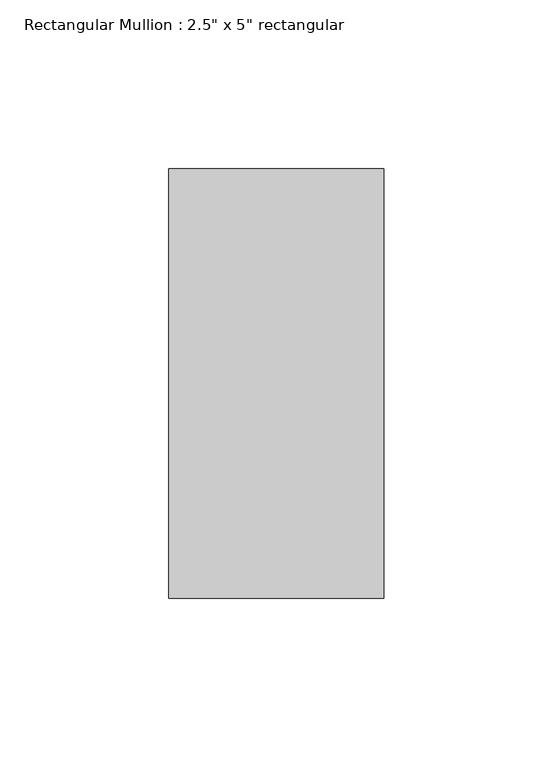
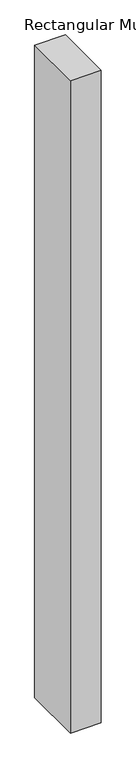
"""IFC4 building model written with IfcOpenShell, lengths in millimetres: member geometry."""

from ifc_helpers import new_model, si_unit, frame, origin, place, context, project, spatial, polyline, outline, extrude, source, transform, mapped, element, save


def member_614527b7(model_context):
    return source(origin(), model_context, "Body", "SweptSolid", [
        extrude(outline(polyline([(0.0, 63.5), (0.0, -63.5), (-63.5, -63.5), (-63.5, 63.5), (0.0, 63.5)])), frame((0.0, 0.0, -1419.063107), z_axis=(0.0, 0.0, 1.0), x_axis=(1.0, 0.0, 0.0)), (0.0, 0.0, 1.0), 1419.063107),
    ])


if __name__ == "__main__":
    model = new_model("IFC4")
    model_context = context("Model", 3, world=origin())
    ifc_project = project(units=[si_unit("LENGTHUNIT", "METRE", prefix="MILLI")], contexts=[model_context])
    site = spatial("IfcSite", under=ifc_project)
    building = spatial("IfcBuilding", under=site)
    placement = place(None, origin())
    member_shape = member_614527b7(model_context)
    element("IfcMember", 1, ObjectType="Rectangular Mullion : 2.5\" x 5\" rectangular", at=placement, inside=building, context=model_context, shape_type="MappedRepresentation", body=[
        mapped(member_shape, transform((0.0, 0.0, 0.0), x_axis=(1.0, 0.0, 0.0), y_axis=(0.0, 1.0, 0.0), z_axis=(0.0, 0.0, 1.0))),
    ])
    save(model, "model.ifc")

# Revit data of these elements
# Type "Rectangular Mullion : 2.5\" x 5\" rectangular"
#   built-in parameter 1007304 = 0.416667 (stored number, unit not read)
#   built-in parameter 1007301 = 0.104167 (stored number, unit not read)
#   built-in parameter 1007300 = 0.104167 (stored number, unit not read)
# Element 1 (IfcMember, "Rectangular Mullion : 2.5\" x 5\" rectangular")
#   Materials on its faces: "Aluminum"
# Materials
#   "Aluminum": class "Metal", colour RGB 247 247 247, transparency 0, Description = "Aluminum 6061", Cost = 0
